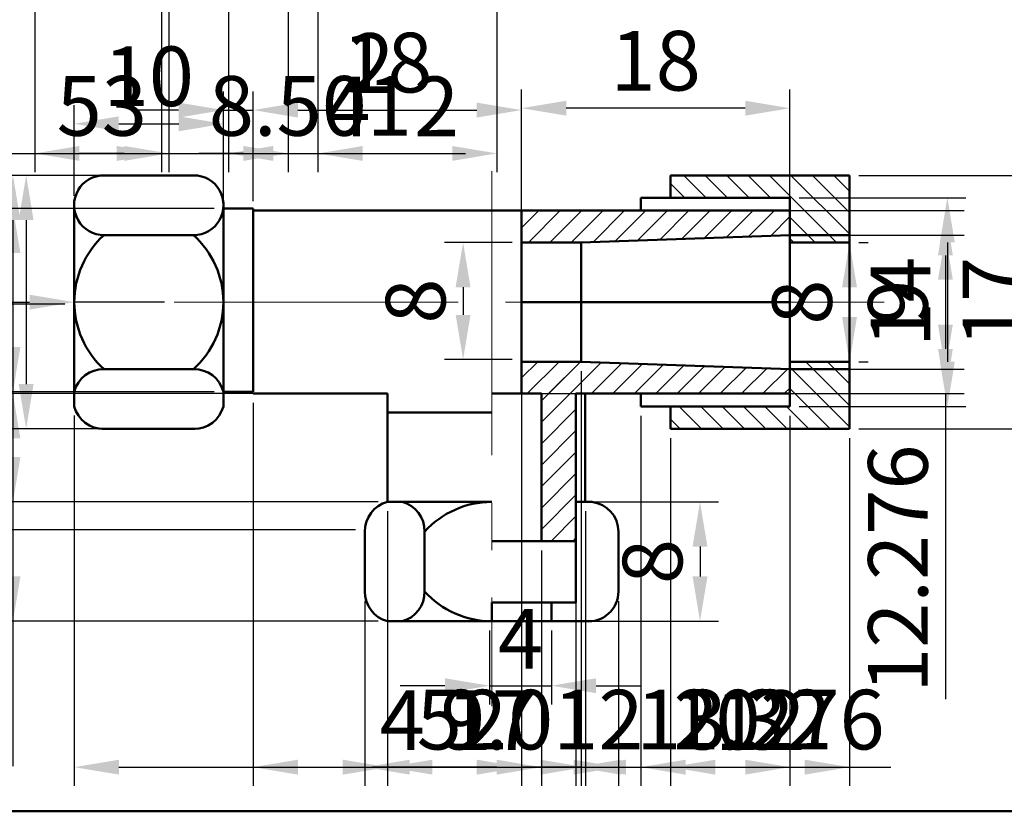
# Model space of a CAD drawing. Units: millimetres. Extents: x 139 to 291, y 28 to 164.
# Tile 2 of 5: x 174 to 240, y 28 to 81. Entities that reach past the tile are written whole.
import ezdxf

# ---------------------------------------------------------------- set-up
doc = ezdxf.new("R2010")
doc.units = ezdxf.units.MM
doc.linetypes.add('CENTER2', pattern=[28.575, 19.05, -3.175, 3.175, -3.175])
for name, color, linetype, lineweight in [('M-CNTR', 1, 'CENTER2', 18), ('M-DIMS', 2, 'Continuous', 25), ('M-HATC', 8, 'Continuous', 18), ('M-OUTL', 7, 'Continuous', 50)]:
    doc.layers.add(name, color=color, linetype=linetype, lineweight=lineweight)
doc.styles.get("Standard").update_dxf_attribs({"font": 'arial.ttf'})
doc.dimstyles.new('ISO-25', dxfattribs={"dimtxt": 4, "dimasz": 3, "dimexe": 1.25, "dimexo": 0.625, "dimtad": 1, "dimdec": 0, "dimtxsty": 'Standard', "dimcen": 2.5, "dimadec": 0, "dimazin": 0, "dimtfac": 1, "dimtdec": 0, "dimtmove": 0, "dimatfit": 3, "dimfxl": 1, "dimarcsym": 0})
pattern_1 = [(45, (183.714, -20.9195), (-0.71842, 0.71842), [])]

# ---------------------------------------------------------------- blocks, each defined once
blk = doc.blocks.new('*D26')
at = {"layer": 'Defpoints', "color": 0, "transparency": 16777216}
for p in [(187.298, 74.293), (177.276, 68.836), (187.298, 68.836)]:
    blk.add_point(p, dxfattribs=at)
at = {"layer": 'M-DIMS', "color": 0, "lineweight": -2, "transparency": 16777216}
for p, q in [((177.276, 69.461), (177.276, 75.543)), ((187.298, 69.461), (187.298, 75.543)), ((180.276, 74.293), (184.298, 74.293))]:
    blk.add_line(p, q, dxfattribs=at)
at = {"layer": 'M-DIMS', "color": 0, "transparency": 16777216}
for points in [[(180.276, 74.793), (180.276, 73.793), (177.276, 74.293)], [(184.298, 74.793), (184.298, 73.793), (187.298, 74.293)]]:
    blk.add_solid(points, dxfattribs=at)
at = {"layer": 'M-DIMS', "color": 0, "transparency": 16777216, "insert": (182.287, 76.96), "char_height": 4, "attachment_point": 5}
blk.add_mtext('10', dxfattribs=at)
blk = doc.blocks.new('*D27')
at = {"layer": 'Defpoints', "color": 0, "transparency": 16777216}
for p in [(180.776, 70.836), (174.061, 53.836), (180.776, 53.836)]:
    blk.add_point(p, dxfattribs=at)
at = {"layer": 'M-DIMS', "color": 0, "lineweight": -2, "transparency": 16777216}
for p, q in [((180.151, 70.836), (172.811, 70.836)), ((174.061, 67.836), (174.061, 56.836)), ((180.151, 53.836), (172.811, 53.836))]:
    blk.add_line(p, q, dxfattribs=at)
at = {"layer": 'M-DIMS', "color": 0, "transparency": 16777216}
for points in [[(173.561, 67.836), (174.561, 67.836), (174.061, 70.836)], [(173.561, 56.836), (174.561, 56.836), (174.061, 53.836)]]:
    blk.add_solid(points, dxfattribs=at)
at = {"layer": 'M-DIMS', "color": 0, "transparency": 16777216, "insert": (171.428, 62.336), "char_height": 4, "attachment_point": 5, "rotation": 90}
blk.add_mtext('17', dxfattribs=at)
blk = doc.blocks.new('*D28')
at = {"layer": 'Defpoints', "color": 0, "transparency": 16777216}
for p in [(177.287, 62.199), (167.49, 47.061), (196.787, 47.061)]:
    blk.add_point(p, dxfattribs=at)
at = {"layer": 'M-DIMS', "color": 0, "lineweight": -2, "transparency": 16777216}
for p, q in [((176.662, 62.199), (166.24, 62.199)), ((167.49, 59.199), (167.49, 50.061)), ((196.162, 47.061), (166.24, 47.061))]:
    blk.add_line(p, q, dxfattribs=at)
at = {"layer": 'M-DIMS', "color": 0, "transparency": 16777216}
for points in [[(166.99, 59.199), (167.99, 59.199), (167.49, 62.199)], [(166.99, 50.061), (167.99, 50.061), (167.49, 47.061)]]:
    blk.add_solid(points, dxfattribs=at)
at = {"layer": 'M-DIMS', "color": 0, "transparency": 16777216, "insert": (164.822, 54.63), "char_height": 4, "attachment_point": 5, "rotation": 90}
blk.add_mtext('15', dxfattribs=at)
blk = doc.blocks.new('*D29')
at = {"layer": 'Defpoints', "color": 0, "transparency": 16777216}
for p in [(211.561, 48.942), (211.469, 40.942), (219.258, 40.942)]:
    blk.add_point(p, dxfattribs=at)
at = {"layer": 'M-DIMS', "color": 0, "lineweight": -2, "transparency": 16777216}
for p, q in [((212.186, 48.942), (220.508, 48.942)), ((219.258, 45.942), (219.258, 43.942)), ((212.094, 40.942), (220.508, 40.942))]:
    blk.add_line(p, q, dxfattribs=at)
at = {"layer": 'M-DIMS', "color": 0, "transparency": 16777216}
for points in [[(218.758, 45.942), (219.758, 45.942), (219.258, 48.942)], [(218.758, 43.942), (219.758, 43.942), (219.258, 40.942)]]:
    blk.add_solid(points, dxfattribs=at)
at = {"layer": 'M-DIMS', "color": 0, "transparency": 16777216, "insert": (216.591, 44.942), "char_height": 4, "attachment_point": 5, "rotation": 90}
blk.add_mtext('8', dxfattribs=at)
blk = doc.blocks.new('*D30')
at = {"layer": 'Defpoints', "color": 0, "transparency": 16777216}
for p in [(205.149, 40.942), (209.287, 40.942), (209.287, 36.614)]:
    blk.add_point(p, dxfattribs=at)
at = {"layer": 'M-DIMS', "color": 0, "lineweight": -2, "transparency": 16777216}
for p, q in [((205.149, 40.317), (205.149, 35.364)), ((209.287, 40.317), (209.287, 35.364)), ((202.149, 36.614), (199.149, 36.614)), ((205.149, 36.614), (209.287, 36.614)), ((212.287, 36.614), (215.287, 36.614))]:
    blk.add_line(p, q, dxfattribs=at)
at = {"layer": 'M-DIMS', "color": 0, "transparency": 16777216}
for points in [[(202.149, 37.114), (202.149, 36.114), (205.149, 36.614)], [(212.287, 37.114), (212.287, 36.114), (209.287, 36.614)]]:
    blk.add_solid(points, dxfattribs=at)
at = {"layer": 'M-DIMS', "color": 0, "transparency": 16777216, "insert": (207.218, 39.239), "char_height": 4, "attachment_point": 5}
blk.add_mtext('4', dxfattribs=at)
blk = doc.blocks.new('*D31')
at = {"layer": 'Defpoints', "color": 0, "transparency": 16777216}
for p in [(229.287, 70.836), (229.287, 53.836), (242.032, 53.836)]:
    blk.add_point(p, dxfattribs=at)
at = {"layer": 'M-DIMS', "color": 0, "lineweight": -2, "transparency": 16777216}
for p, q in [((229.912, 70.836), (243.282, 70.836)), ((242.032, 67.836), (242.032, 56.836)), ((229.912, 53.836), (243.282, 53.836))]:
    blk.add_line(p, q, dxfattribs=at)
at = {"layer": 'M-DIMS', "color": 0, "transparency": 16777216}
for points in [[(241.532, 67.836), (242.532, 67.836), (242.032, 70.836)], [(241.532, 56.836), (242.532, 56.836), (242.032, 53.836)]]:
    blk.add_solid(points, dxfattribs=at)
at = {"layer": 'M-DIMS', "color": 0, "transparency": 16777216, "insert": (239.399, 62.336), "char_height": 4, "attachment_point": 5, "rotation": 90}
blk.add_mtext('17', dxfattribs=at)
blk = doc.blocks.new('*D32')
at = {"layer": 'Defpoints', "color": 0, "transparency": 16777216}
for p in [(225.287, 69.336), (225.287, 55.336), (235.847, 55.336)]:
    blk.add_point(p, dxfattribs=at)
at = {"layer": 'M-DIMS', "color": 0, "lineweight": -2, "transparency": 16777216}
for p, q in [((225.912, 69.336), (237.097, 69.336)), ((235.847, 66.336), (235.847, 58.336)), ((225.912, 55.336), (237.097, 55.336))]:
    blk.add_line(p, q, dxfattribs=at)
at = {"layer": 'M-DIMS', "color": 0, "transparency": 16777216}
for points in [[(235.347, 66.336), (236.347, 66.336), (235.847, 69.336)], [(235.347, 58.336), (236.347, 58.336), (235.847, 55.336)]]:
    blk.add_solid(points, dxfattribs=at)
at = {"layer": 'M-DIMS', "color": 0, "transparency": 16777216, "insert": (233.214, 62.336), "char_height": 4, "attachment_point": 5, "rotation": 90}
blk.add_mtext('14', dxfattribs=at)
blk = doc.blocks.new('*D33')
at = {"layer": 'Defpoints', "color": 0, "transparency": 16777216}
for p in [(229.287, 66.336), (229.287, 58.336), (229.287, 58.336)]:
    blk.add_point(p, dxfattribs=at)
at = {"layer": 'M-DIMS', "color": 0, "lineweight": -2, "transparency": 16777216}
for p, q in [((229.912, 66.336), (230.537, 66.336)), ((229.287, 63.336), (229.287, 61.336)), ((229.912, 58.336), (230.537, 58.336))]:
    blk.add_line(p, q, dxfattribs=at)
at = {"layer": 'M-DIMS', "color": 0, "transparency": 16777216}
for points in [[(228.787, 63.336), (229.787, 63.336), (229.287, 66.336)], [(228.787, 61.336), (229.787, 61.336), (229.287, 58.336)]]:
    blk.add_solid(points, dxfattribs=at)
at = {"layer": 'M-DIMS', "color": 0, "transparency": 16777216, "insert": (226.62, 62.336), "char_height": 4, "attachment_point": 5, "rotation": 90}
blk.add_mtext('8', dxfattribs=at)
blk = doc.blocks.new('*D34')
at = {"layer": 'Defpoints', "color": 0, "transparency": 16777216}
for p in [(207.287, 66.336), (203.367, 58.479), (207.287, 58.479)]:
    blk.add_point(p, dxfattribs=at)
at = {"layer": 'M-DIMS', "color": 0, "lineweight": -2, "transparency": 16777216}
for p, q in [((206.662, 66.336), (202.117, 66.336)), ((203.367, 63.336), (203.367, 61.479)), ((206.662, 58.479), (202.117, 58.479))]:
    blk.add_line(p, q, dxfattribs=at)
at = {"layer": 'M-DIMS', "color": 0, "transparency": 16777216}
for points in [[(202.867, 63.336), (203.867, 63.336), (203.367, 66.336)], [(202.867, 61.479), (203.867, 61.479), (203.367, 58.479)]]:
    blk.add_solid(points, dxfattribs=at)
at = {"layer": 'M-DIMS', "color": 0, "transparency": 16777216, "insert": (200.7, 62.408), "char_height": 4, "attachment_point": 5, "rotation": 90}
blk.add_mtext('8', dxfattribs=at)
blk = doc.blocks.new('*D35')
at = {"layer": 'Defpoints', "color": 0, "transparency": 16777216}
for p in [(207.287, 75.339), (207.287, 62.336), (225.287, 62.336)]:
    blk.add_point(p, dxfattribs=at)
at = {"layer": 'M-DIMS', "color": 0, "lineweight": -2, "transparency": 16777216}
for p, q in [((207.287, 62.961), (207.287, 76.589)), ((225.287, 62.961), (225.287, 76.589)), ((222.287, 75.339), (210.287, 75.339))]:
    blk.add_line(p, q, dxfattribs=at)
at = {"layer": 'M-DIMS', "color": 0, "transparency": 16777216}
for points in [[(210.287, 75.839), (210.287, 74.839), (207.287, 75.339)], [(222.287, 75.839), (222.287, 74.839), (225.287, 75.339)]]:
    blk.add_solid(points, dxfattribs=at)
at = {"layer": 'M-DIMS', "color": 0, "transparency": 16777216, "insert": (216.287, 78.006), "char_height": 4, "attachment_point": 5}
blk.add_mtext('18', dxfattribs=at)
blk = doc.blocks.new('*D36')
at = {"layer": 'Defpoints', "color": 0, "transparency": 16777216}
for p in [(152.636, 94.663), (205.636, 89.163), (205.636, 72.308)]:
    blk.add_point(p, dxfattribs=at)
at = {"layer": 'M-DIMS', "color": 0, "lineweight": -2, "transparency": 16777216}
for p, q in [((152.636, 94.038), (152.636, 71.058)), ((205.636, 88.538), (205.636, 71.058)), ((155.636, 72.308), (202.636, 72.308))]:
    blk.add_line(p, q, dxfattribs=at)
at = {"layer": 'M-DIMS', "color": 0, "transparency": 16777216}
for points in [[(155.636, 72.808), (155.636, 71.808), (152.636, 72.308)], [(202.636, 72.808), (202.636, 71.808), (205.636, 72.308)]]:
    blk.add_solid(points, dxfattribs=at)
at = {"layer": 'M-DIMS', "color": 0, "transparency": 16777216, "insert": (179.136, 74.977), "char_height": 4, "attachment_point": 5}
blk.add_mtext('53', dxfattribs=at)
blk = doc.blocks.new('*D37')
at = {"layer": 'Defpoints', "color": 0, "transparency": 16777216}
for p in [(174.636, 99.163), (183.137, 99.163), (183.137, 72.308)]:
    blk.add_point(p, dxfattribs=at)
at = {"layer": 'M-DIMS', "color": 0, "lineweight": -2, "transparency": 16777216}
for p, q in [((174.636, 98.538), (174.636, 71.058)), ((183.137, 98.538), (183.137, 71.058)), ((177.636, 72.308), (180.137, 72.308)), ((183.137, 72.308), (200.118, 72.308))]:
    blk.add_line(p, q, dxfattribs=at)
at = {"layer": 'M-DIMS', "color": 0, "transparency": 16777216}
for points in [[(177.636, 72.808), (177.636, 71.808), (174.636, 72.308)], [(180.137, 72.808), (180.137, 71.808), (183.137, 72.308)]]:
    blk.add_solid(points, dxfattribs=at)
at = {"layer": 'M-DIMS', "color": 0, "transparency": 16777216, "insert": (193.128, 74.976), "char_height": 4, "attachment_point": 5}
blk.add_mtext('8.501', dxfattribs=at)
blk = doc.blocks.new('*D38')
at = {"layer": 'Defpoints', "color": 0, "transparency": 16777216}
for p in [(187.636, 101.663), (183.636, 97.663), (187.636, 72.308)]:
    blk.add_point(p, dxfattribs=at)
at = {"layer": 'M-DIMS', "color": 0, "lineweight": -2, "transparency": 16777216}
for p, q in [((187.636, 101.038), (187.636, 71.058)), ((183.636, 97.038), (183.636, 71.058)), ((180.636, 72.308), (177.636, 72.308)), ((183.636, 72.308), (187.636, 72.308)), ((190.636, 72.308), (197.653, 72.308))]:
    blk.add_line(p, q, dxfattribs=at)
at = {"layer": 'M-DIMS', "color": 0, "transparency": 16777216}
for points in [[(180.636, 72.808), (180.636, 71.808), (183.636, 72.308)], [(190.636, 72.808), (190.636, 71.808), (187.636, 72.308)]]:
    blk.add_solid(points, dxfattribs=at)
at = {"layer": 'M-DIMS', "color": 0, "transparency": 16777216, "insert": (195.644, 74.933), "char_height": 4, "attachment_point": 5}
blk.add_mtext('4', dxfattribs=at)
blk = doc.blocks.new('*D41')
at = {"layer": 'Defpoints', "color": 0, "transparency": 16777216}
for p in [(191.636, 104.663), (193.636, 104.663), (193.636, 72.308)]:
    blk.add_point(p, dxfattribs=at)
at = {"layer": 'M-DIMS', "color": 0, "lineweight": -2, "transparency": 16777216}
for p, q in [((191.636, 104.038), (191.636, 71.058)), ((193.636, 104.038), (193.636, 71.058)), ((188.636, 72.308), (185.636, 72.308)), ((191.636, 72.308), (193.636, 72.308)), ((196.636, 72.308), (203.535, 72.308))]:
    blk.add_line(p, q, dxfattribs=at)
at = {"layer": 'M-DIMS', "color": 0, "transparency": 16777216}
for points in [[(188.636, 72.808), (188.636, 71.808), (191.636, 72.308)], [(196.636, 72.808), (196.636, 71.808), (193.636, 72.308)]]:
    blk.add_solid(points, dxfattribs=at)
at = {"layer": 'M-DIMS', "color": 0, "transparency": 16777216, "insert": (201.586, 74.942), "char_height": 4, "attachment_point": 5}
blk.add_mtext('2', dxfattribs=at)
blk = doc.blocks.new('*D42')
at = {"layer": 'Defpoints', "color": 0, "transparency": 16777216}
for p in [(177.287, 55.349), (229.287, 53.836), (229.287, 31.154)]:
    blk.add_point(p, dxfattribs=at)
at = {"layer": 'M-DIMS', "color": 0, "lineweight": -2, "transparency": 16777216}
for p, q in [((177.287, 54.724), (177.287, 29.904)), ((229.287, 53.211), (229.287, 29.904)), ((180.287, 31.154), (226.287, 31.154))]:
    blk.add_line(p, q, dxfattribs=at)
at = {"layer": 'M-DIMS', "color": 0, "transparency": 16777216}
for points in [[(180.287, 31.654), (180.287, 30.654), (177.287, 31.154)], [(226.287, 31.654), (226.287, 30.654), (229.287, 31.154)]]:
    blk.add_solid(points, dxfattribs=at)
at = {"layer": 'M-DIMS', "color": 0, "transparency": 16777216, "insert": (203.287, 33.822), "char_height": 4, "attachment_point": 5}
blk.add_mtext('52', dxfattribs=at)
blk = doc.blocks.new('*D43')
at = {"layer": 'Defpoints', "color": 0, "transparency": 16777216}
for p in [(179.287, 70.836), (173.176, 40.942), (198.299, 40.942)]:
    blk.add_point(p, dxfattribs=at)
at = {"layer": 'M-DIMS', "color": 0, "lineweight": -2, "transparency": 16777216}
for p, q in [((178.662, 70.836), (171.926, 70.836)), ((173.176, 67.836), (173.176, 43.942)), ((197.674, 40.942), (171.926, 40.942))]:
    blk.add_line(p, q, dxfattribs=at)
at = {"layer": 'M-DIMS', "color": 0, "transparency": 16777216}
for points in [[(172.676, 67.836), (173.676, 67.836), (173.176, 70.836)], [(172.676, 43.942), (173.676, 43.942), (173.176, 40.942)]]:
    blk.add_solid(points, dxfattribs=at)
at = {"layer": 'M-DIMS', "color": 0, "transparency": 16777216, "insert": (170.509, 55.889), "char_height": 4, "attachment_point": 5, "rotation": 90}
blk.add_mtext('29.895', dxfattribs=at)
blk = doc.blocks.new('*D44')
at = {"layer": 'Defpoints', "color": 0, "transparency": 16777216}
for p in [(207.287, 68.474), (207.287, 56.199), (235.718, 56.199)]:
    blk.add_point(p, dxfattribs=at)
at = {"layer": 'M-DIMS', "color": 0, "lineweight": -2, "transparency": 16777216}
for p, q in [((207.912, 68.474), (236.968, 68.474)), ((235.718, 65.474), (235.718, 59.199)), ((207.912, 56.199), (236.968, 56.199)), ((235.718, 56.199), (235.718, 35.722))]:
    blk.add_line(p, q, dxfattribs=at)
at = {"layer": 'M-DIMS', "color": 0, "transparency": 16777216}
for points in [[(235.218, 65.474), (236.218, 65.474), (235.718, 68.474)], [(235.218, 59.199), (236.218, 59.199), (235.718, 56.199)]]:
    blk.add_solid(points, dxfattribs=at)
at = {"layer": 'M-DIMS', "color": 0, "transparency": 16777216, "insert": (233.051, 44.46), "char_height": 4, "attachment_point": 5, "rotation": 90}
blk.add_mtext('12.276', dxfattribs=at)
blk = doc.blocks.new('*D45')
at = {"layer": 'Defpoints', "color": 0, "transparency": 16777216}
for p in [(189.287, 75.214), (187.287, 68.624), (189.287, 68.624)]:
    blk.add_point(p, dxfattribs=at)
at = {"layer": 'M-DIMS', "color": 0, "lineweight": -2, "transparency": 16777216}
for p, q in [((187.287, 69.249), (187.287, 76.464)), ((189.287, 69.249), (189.287, 76.464)), ((184.287, 75.214), (181.287, 75.214)), ((187.287, 75.214), (189.287, 75.214)), ((192.287, 75.214), (199.187, 75.214))]:
    blk.add_line(p, q, dxfattribs=at)
at = {"layer": 'M-DIMS', "color": 0, "transparency": 16777216}
for points in [[(184.287, 75.714), (184.287, 74.714), (187.287, 75.214)], [(192.287, 75.714), (192.287, 74.714), (189.287, 75.214)]]:
    blk.add_solid(points, dxfattribs=at)
at = {"layer": 'M-DIMS', "color": 0, "transparency": 16777216, "insert": (197.237, 77.847), "char_height": 4, "attachment_point": 5}
blk.add_mtext('2', dxfattribs=at)
blk = doc.blocks.new('*D46')
at = {"layer": 'Defpoints', "color": 0, "transparency": 16777216}
for p in [(187.287, 68.624), (173.176, 56.324), (187.287, 56.324)]:
    blk.add_point(p, dxfattribs=at)
at = {"layer": 'M-DIMS', "color": 0, "lineweight": -2, "transparency": 16777216}
for p, q in [((186.662, 68.624), (171.926, 68.624)), ((173.176, 65.624), (173.176, 59.324)), ((186.662, 56.324), (171.926, 56.324))]:
    blk.add_line(p, q, dxfattribs=at)
at = {"layer": 'M-DIMS', "color": 0, "transparency": 16777216}
for points in [[(172.676, 65.624), (173.676, 65.624), (173.176, 68.624)], [(172.676, 59.324), (173.676, 59.324), (173.176, 56.324)]]:
    blk.add_solid(points, dxfattribs=at)
at = {"layer": 'M-DIMS', "color": 0, "transparency": 16777216, "insert": (170.507, 62.474), "char_height": 4, "attachment_point": 5, "rotation": 90}
blk.add_mtext('12.3', dxfattribs=at)
blk = doc.blocks.new('*D47')
at = {"layer": 'Defpoints', "color": 0, "transparency": 16777216}
for p in [(207.287, 75.214), (189.287, 68.474), (207.287, 68.474)]:
    blk.add_point(p, dxfattribs=at)
at = {"layer": 'M-DIMS', "color": 0, "lineweight": -2, "transparency": 16777216}
for p, q in [((189.287, 69.099), (189.287, 76.464)), ((207.287, 69.099), (207.287, 76.464)), ((192.287, 75.214), (204.287, 75.214))]:
    blk.add_line(p, q, dxfattribs=at)
at = {"layer": 'M-DIMS', "color": 0, "transparency": 16777216}
for points in [[(192.287, 75.714), (192.287, 74.714), (189.287, 75.214)], [(204.287, 75.714), (204.287, 74.714), (207.287, 75.214)]]:
    blk.add_solid(points, dxfattribs=at)
at = {"layer": 'M-DIMS', "color": 0, "transparency": 16777216, "insert": (198.287, 77.881), "char_height": 4, "attachment_point": 5}
blk.add_mtext('18', dxfattribs=at)
blk = doc.blocks.new('*D48')
at = {"layer": 'Defpoints', "color": 0, "transparency": 16777216}
for p in [(189.287, 56.199), (198.299, 48.942), (198.299, 31.154)]:
    blk.add_point(p, dxfattribs=at)
at = {"layer": 'M-DIMS', "color": 0, "lineweight": -2, "transparency": 16777216}
for p, q in [((189.287, 55.574), (189.287, 29.904)), ((198.299, 48.317), (198.299, 29.904)), ((192.287, 31.154), (195.299, 31.154)), ((198.299, 31.154), (216.006, 31.154))]:
    blk.add_line(p, q, dxfattribs=at)
at = {"layer": 'M-DIMS', "color": 0, "transparency": 16777216}
for points in [[(192.287, 31.654), (192.287, 30.654), (189.287, 31.154)], [(195.299, 31.654), (195.299, 30.654), (198.299, 31.154)]]:
    blk.add_solid(points, dxfattribs=at)
at = {"layer": 'M-DIMS', "color": 0, "transparency": 16777216, "insert": (208.653, 33.822), "char_height": 4, "attachment_point": 5}
blk.add_mtext('9.012', dxfattribs=at)
blk = doc.blocks.new('*D49')
at = {"layer": 'Defpoints', "color": 0, "transparency": 16777216}
for p in [(198.299, 48.942), (211.575, 48.942), (211.575, 31.154)]:
    blk.add_point(p, dxfattribs=at)
at = {"layer": 'M-DIMS', "color": 0, "lineweight": -2, "transparency": 16777216}
for p, q in [((198.299, 48.317), (198.299, 29.904)), ((211.575, 48.317), (211.575, 29.904)), ((201.299, 31.154), (208.575, 31.154)), ((211.575, 31.154), (232.051, 31.154))]:
    blk.add_line(p, q, dxfattribs=at)
at = {"layer": 'M-DIMS', "color": 0, "transparency": 16777216}
for points in [[(201.299, 31.654), (201.299, 30.654), (198.299, 31.154)], [(208.575, 31.654), (208.575, 30.654), (211.575, 31.154)]]:
    blk.add_solid(points, dxfattribs=at)
at = {"layer": 'M-DIMS', "color": 0, "transparency": 16777216, "insert": (223.313, 33.823), "char_height": 4, "attachment_point": 5}
blk.add_mtext('13.276', dxfattribs=at)
blk = doc.blocks.new('*D50')
at = {"layer": 'Defpoints', "color": 0, "transparency": 16777216}
for p in [(198.299, 56.199), (173.176, 48.942), (198.299, 48.942)]:
    blk.add_point(p, dxfattribs=at)
at = {"layer": 'M-DIMS', "color": 0, "lineweight": -2, "transparency": 16777216}
for p, q in [((197.674, 56.199), (171.926, 56.199)), ((173.176, 53.199), (173.176, 51.942)), ((197.674, 48.942), (171.926, 48.942)), ((173.176, 48.942), (173.176, 31.227))]:
    blk.add_line(p, q, dxfattribs=at)
at = {"layer": 'M-DIMS', "color": 0, "transparency": 16777216}
for points in [[(172.676, 53.199), (173.676, 53.199), (173.176, 56.199)], [(172.676, 51.942), (173.676, 51.942), (173.176, 48.942)]]:
    blk.add_solid(points, dxfattribs=at)
at = {"layer": 'M-DIMS', "color": 0, "transparency": 16777216, "insert": (170.509, 38.584), "char_height": 4, "attachment_point": 5, "rotation": 90}
blk.add_mtext('7.257', dxfattribs=at)
blk = doc.blocks.new('*D51')
at = {"layer": 'Defpoints', "color": 0, "transparency": 16777216}
for p in [(196.787, 42.942), (213.787, 42.919), (213.787, 31.154)]:
    blk.add_point(p, dxfattribs=at)
at = {"layer": 'M-DIMS', "color": 0, "lineweight": -2, "transparency": 16777216}
for p, q in [((196.787, 42.317), (196.787, 29.904)), ((213.787, 42.294), (213.787, 29.904)), ((199.787, 31.154), (210.787, 31.154))]:
    blk.add_line(p, q, dxfattribs=at)
at = {"layer": 'M-DIMS', "color": 0, "transparency": 16777216}
for points in [[(199.787, 31.654), (199.787, 30.654), (196.787, 31.154)], [(210.787, 31.654), (210.787, 30.654), (213.787, 31.154)]]:
    blk.add_solid(points, dxfattribs=at)
at = {"layer": 'M-DIMS', "color": 0, "transparency": 16777216, "insert": (205.287, 33.788), "char_height": 4, "attachment_point": 5}
blk.add_mtext('17', dxfattribs=at)
blk = doc.blocks.new('*D52')
at = {"layer": 'Defpoints', "color": 0, "transparency": 16777216}
for p in [(208.623, 46.316), (210.938, 46.316), (210.938, 31.154)]:
    blk.add_point(p, dxfattribs=at)
at = {"layer": 'M-DIMS', "color": 0, "lineweight": -2, "transparency": 16777216}
for p, q in [((208.623, 45.691), (208.623, 29.904)), ((210.938, 45.691), (210.938, 29.904)), ((205.623, 31.154), (202.623, 31.154)), ((208.623, 31.154), (210.938, 31.154)), ((213.938, 31.154), (228.606, 31.154))]:
    blk.add_line(p, q, dxfattribs=at)
at = {"layer": 'M-DIMS', "color": 0, "transparency": 16777216}
for points in [[(205.623, 31.654), (205.623, 30.654), (208.623, 31.154)], [(213.938, 31.654), (213.938, 30.654), (210.938, 31.154)]]:
    blk.add_solid(points, dxfattribs=at)
at = {"layer": 'M-DIMS', "color": 0, "transparency": 16777216, "insert": (222.772, 33.823), "char_height": 4, "attachment_point": 5}
blk.add_mtext('2.32', dxfattribs=at)
blk = doc.blocks.new('*D53')
at = {"layer": 'Defpoints', "color": 0, "transparency": 16777216}
for p in [(215.287, 55.336), (225.287, 55.336), (225.287, 31.154)]:
    blk.add_point(p, dxfattribs=at)
at = {"layer": 'M-DIMS', "color": 0, "lineweight": -2, "transparency": 16777216}
for p, q in [((215.287, 54.711), (215.287, 29.904)), ((225.287, 54.711), (225.287, 29.904)), ((218.287, 31.154), (222.287, 31.154))]:
    blk.add_line(p, q, dxfattribs=at)
at = {"layer": 'M-DIMS', "color": 0, "transparency": 16777216}
for points in [[(218.287, 31.654), (218.287, 30.654), (215.287, 31.154)], [(222.287, 31.654), (222.287, 30.654), (225.287, 31.154)]]:
    blk.add_solid(points, dxfattribs=at)
at = {"layer": 'M-DIMS', "color": 0, "transparency": 16777216, "insert": (220.287, 33.822), "char_height": 4, "attachment_point": 5}
blk.add_mtext('10', dxfattribs=at)
blk = doc.blocks.new('*D54')
at = {"layer": 'Defpoints', "color": 0, "transparency": 16777216}
for p in [(217.287, 53.836), (229.287, 53.836), (229.287, 31.154)]:
    blk.add_point(p, dxfattribs=at)
at = {"layer": 'M-DIMS', "color": 0, "lineweight": -2, "transparency": 16777216}
for p, q in [((217.287, 53.211), (217.287, 29.904)), ((229.287, 53.211), (229.287, 29.904)), ((220.287, 31.154), (226.287, 31.154))]:
    blk.add_line(p, q, dxfattribs=at)
at = {"layer": 'M-DIMS', "color": 0, "transparency": 16777216}
for points in [[(220.287, 31.654), (220.287, 30.654), (217.287, 31.154)], [(226.287, 31.654), (226.287, 30.654), (229.287, 31.154)]]:
    blk.add_solid(points, dxfattribs=at)
at = {"layer": 'M-DIMS', "color": 0, "transparency": 16777216, "insert": (223.287, 33.788), "char_height": 4, "attachment_point": 5}
blk.add_mtext('12', dxfattribs=at)
blk = doc.blocks.new('*D55')
at = {"layer": 'Defpoints', "color": 0, "transparency": 16777216}
for p in [(207.287, 58.336), (211.287, 58.336), (207.287, 31.154)]:
    blk.add_point(p, dxfattribs=at)
at = {"layer": 'M-DIMS', "color": 0, "lineweight": -2, "transparency": 16777216}
for p, q in [((207.287, 57.711), (207.287, 29.904)), ((211.287, 57.711), (211.287, 29.904)), ((204.287, 31.154), (197.27, 31.154)), ((211.287, 31.154), (207.287, 31.154)), ((214.287, 31.154), (217.287, 31.154))]:
    blk.add_line(p, q, dxfattribs=at)
at = {"layer": 'M-DIMS', "color": 0, "transparency": 16777216}
for points in [[(204.287, 31.654), (204.287, 30.654), (207.287, 31.154)], [(214.287, 31.654), (214.287, 30.654), (211.287, 31.154)]]:
    blk.add_solid(points, dxfattribs=at)
at = {"layer": 'M-DIMS', "color": 0, "transparency": 16777216, "insert": (199.279, 33.779), "char_height": 4, "attachment_point": 5}
blk.add_mtext('4', dxfattribs=at)
blk = doc.blocks.new('*D56')
at = {"layer": 'Defpoints', "color": 0, "transparency": 16777216}
for p in [(225.287, 66.836), (225.287, 57.836), (235.718, 57.836)]:
    blk.add_point(p, dxfattribs=at)
at = {"layer": 'M-DIMS', "color": 0, "lineweight": -2, "transparency": 16777216}
for p, q in [((225.912, 66.836), (236.968, 66.836)), ((235.718, 63.836), (235.718, 60.836)), ((225.912, 57.836), (236.968, 57.836))]:
    blk.add_line(p, q, dxfattribs=at)
at = {"layer": 'M-DIMS', "color": 0, "transparency": 16777216}
for points in [[(235.218, 63.836), (236.218, 63.836), (235.718, 66.836)], [(235.218, 60.836), (236.218, 60.836), (235.718, 57.836)]]:
    blk.add_solid(points, dxfattribs=at)
at = {"layer": 'M-DIMS', "color": 0, "transparency": 16777216, "insert": (233.051, 62.336), "char_height": 4, "attachment_point": 5, "rotation": 90}
blk.add_mtext('9', dxfattribs=at)
blk = doc.blocks.new('*D60')
at = {"layer": 'Defpoints', "color": 0, "transparency": 16777216}
for p in [(177.287, 62.336), (183.35, 62.336)]:
    blk.add_point(p, dxfattribs=at)
at = {"layer": 'M-DIMS', "color": 0, "lineweight": -2, "transparency": 16777216}
for p, q in [((152.711, 62.334), (174.287, 62.336)), ((183.35, 62.336), (177.287, 62.336))]:
    blk.add_line(p, q, dxfattribs=at)
at = {"layer": 'M-DIMS', "color": 0, "transparency": 16777216}
blk.add_solid([(174.287, 62.836), (174.287, 61.836), (177.287, 62.336)], dxfattribs=at)
at = {"layer": 'M-DIMS', "color": 0, "transparency": 16777216, "insert": (161.999, 65.004), "char_height": 4, "attachment_point": 5, "rotation": 0.00419}
blk.add_mtext('R6.063', dxfattribs=at)

msp = doc.modelspace()

# ---------------------------------------------------------------- hatches: boundary and pattern name
at = {"layer": 'M-HATC'}
h = msp.add_hatch(dxfattribs=at)
h.set_pattern_fill('ANSI31', color=256, scale=0.32, angle=90)
h.set_pattern_definition([(135, (23.6513, -43.5646), (-0.7184205, -0.7184205), [])])
h.paths.add_polyline_path([(229.2871, 70.8364), (217.2871, 70.8364), (217.2871, 69.3364), (225.2871, 69.3364), (225.2871, 66.8364), (229.2871, 66.8364)])
h.paths.add_polyline_path([(229.2871, 66.8364), (225.2871, 66.8364), (225.2871, 66.3364), (229.2871, 66.3364)])
h.paths.add_polyline_path([(229.2871, 57.8364), (225.2871, 57.8364), (225.2871, 55.3364), (217.2871, 55.3364), (217.2871, 53.8364), (229.2871, 53.8364)])
h.paths.add_polyline_path([(229.2871, 58.3364), (225.2871, 58.3364), (225.2871, 57.8364), (229.2871, 57.8364)])
h = msp.add_hatch(dxfattribs=at)
h.set_pattern_fill('ANSI31', color=256, scale=0.32)
h.set_pattern_definition(pattern_1)
h.paths.add_polyline_path([(225.2871, 68.4743), (211.2871, 68.4743), (211.2871, 66.3364), (225.2871, 66.8364)])
h.paths.add_polyline_path([(211.2871, 68.4743), (207.2871, 68.4743), (207.2871, 66.3364), (211.2871, 66.3364)])
h.paths.add_polyline_path([(211.2871, 58.3364), (207.2871, 58.3364), (207.2871, 56.1986), (211.2871, 56.1986)])
h.paths.add_polyline_path([(225.2871, 57.8364), (211.2871, 58.3364), (211.2871, 56.1986), (225.2871, 56.1986)])
h = msp.add_hatch(dxfattribs=at)
h.set_pattern_fill('ANSI31', color=256, scale=0.32)
h.set_pattern_definition(pattern_1)
h.paths.add_polyline_path([(210.9384, 56.1986), (225.2871, 56.1986), (225.2871, 57.8364), (211.2871, 58.3364), (207.2871, 58.3364), (207.2871, 56.1986), (208.6231, 56.1986), (208.6231, 46.3157), (210.9384, 46.3157)])

# ---------------------------------------------------------------- linework, layer by layer
at = {"layer": 'M-CNTR'}
for p, q in [((205.2871, 71.1136), (205.2871, 35.2545)), ((231.6179, 62.3364), (177.2871, 62.3364))]:
    msp.add_line(p, q, dxfattribs=at)
at = {"layer": 'M-OUTL'}
for p, q in [((182.2871, 70.8364), (179.2646, 70.8364)), ((185.3097, 70.8364), (182.2871, 70.8364)), ((217.2871, 69.3364), (217.2871, 70.8364)), ((217.2871, 70.8364), (229.2871, 70.8364)), ((229.2871, 62.3364), (229.2871, 70.8364)), ((177.2871, 69.0487), (177.2871, 55.3485)), ((187.2871, 55.3485), (187.2871, 69.0487)), ((225.2871, 69.3364), (215.2871, 69.3364)), ((215.2871, 69.3364), (215.2871, 68.4743)), ((225.2871, 66.8364), (225.2871, 69.3364)), ((177.2871, 68.1986), (177.3803, 68.1986)), ((187.2871, 68.6242), (189.2871, 68.6242)), ((189.2871, 68.6242), (189.2871, 56.3244)), ((189.2871, 62.4743), (189.2871, 68.4743)), ((189.2871, 68.4743), (225.2871, 68.4743)), ((207.2871, 56.1986), (207.2871, 68.4743)), ((182.2871, 66.8364), (179.2646, 66.8364)), ((185.3097, 66.8364), (182.2871, 66.8364)), ((211.2871, 66.3364), (225.2871, 66.8364)), ((225.2871, 66.8364), (229.2871, 66.8364)), ((225.2871, 66.3364), (225.2871, 66.8364)), ((211.2871, 66.3364), (207.2871, 66.3364)), ((207.2871, 66.3364), (207.2871, 58.4793)), ((211.2871, 62.3364), (211.2871, 66.3364)), ((225.2871, 66.3364), (229.2871, 66.3364)), ((225.2871, 66.3364), (225.2871, 58.3364)), ((225.2871, 62.3364), (207.2871, 62.3364)), ((211.2871, 62.3364), (211.2871, 58.3364)), ((229.2871, 62.3364), (229.2871, 53.8364)), ((211.2871, 58.3364), (207.2871, 58.3364)), ((211.2871, 58.3364), (225.2871, 57.8364)), ((225.2871, 58.3364), (229.2871, 58.3364)), ((225.2871, 57.8364), (225.2871, 58.3364)), ((182.2871, 57.8364), (179.1681, 57.8364)), ((185.4062, 57.8364), (182.2871, 57.8364)), ((225.2871, 57.8364), (229.2871, 57.8364)), ((225.2871, 57.8364), (225.2871, 55.3364)), ((189.2871, 56.3244), (187.2871, 56.3244)), ((189.2871, 56.1986), (198.2992, 56.1986)), ((198.2992, 48.9417), (198.2992, 56.1986)), ((205.2871, 56.1986), (208.6231, 56.1986)), ((208.6231, 56.1986), (208.6231, 46.3157)), ((210.9384, 46.3157), (210.9384, 56.1986)), ((210.9384, 56.1986), (225.2871, 56.1986)), ((211.5607, 48.9401), (211.5607, 56.1986)), ((215.2871, 55.8364), (215.2871, 56.1986)), ((215.2871, 55.3364), (215.2871, 55.8364)), ((198.2992, 54.9417), (205.2871, 54.9417)), ((225.2871, 55.3364), (215.2871, 55.3364)), ((217.2871, 53.8364), (217.2871, 55.3364)), ((179.1681, 53.8364), (182.2871, 53.8364)), ((182.2871, 53.8364), (185.4062, 53.8364)), ((229.2871, 53.8364), (217.2871, 53.8364)), ((205.2871, 48.9417), (198.2992, 48.9417)), ((211.9994, 48.9417), (210.9384, 48.9417)), ((196.7871, 47.0608), (196.7871, 44.9417)), ((200.7871, 44.9417), (200.7871, 47.0607)), ((213.7871, 44.9417), (213.7871, 46.9642)), ((205.2871, 46.3157), (210.9384, 46.3157)), ((210.9384, 46.3157), (210.9384, 42.1853)), ((196.7871, 44.9417), (196.7871, 42.8227)), ((200.7871, 42.8227), (200.7871, 44.9417)), ((213.7871, 42.9192), (213.7871, 44.9417)), ((210.9384, 42.1853), (205.2871, 42.1853)), ((205.2871, 42.1853), (205.2871, 40.9417)), ((209.2871, 42.1853), (209.2871, 40.9417)), ((198.2992, 40.9417), (211.9994, 40.9417)), ((207.2871, 40.9417), (207.2871, 40.9433))]:
    msp.add_line(p, q, dxfattribs=at)
msp.add_lwpolyline([(139.74, 164.2339), (291.244, 164.2339), (291.244, 28.1944), (139.74, 28.1944)], close=True, dxfattribs=at)
for centre, radius, start, end in [((179.2759, 68.8364), 2, 89.677332, 270.322668), ((185.2984, 68.8364), 2, 269.677332, 90.322668), ((183.3496, 62.3364), 6.0625, 132.075022, 227.924978), ((181.2246, 62.3364), 6.0625, 312.075022, 47.924978), ((179.2276, 55.8364), 2.0009, 88.295425, 165.885789), ((185.3467, 55.8364), 2.0009, 14.114211, 91.704575), ((179.2276, 55.8364), 2.0009, 194.114211, 271.70457), ((185.3467, 55.8364), 2.0009, 268.29543, 345.885789), ((198.7871, 47.0012), 2.0009, 104.114211, 181.70457), ((198.7871, 47.0012), 2.0009, 358.295425, 75.885789), ((205.2871, 42.8792), 6.0625, 90, 137.924978), ((211.7871, 46.953), 2, 96.092116, 96.50143), ((211.7871, 46.953), 2, 359.677332, 83.907884), ((198.7871, 42.8822), 2.0009, 178.29543, 255.885789), ((198.7871, 42.8822), 2.0009, 284.114211, 1.704575), ((205.2871, 47.0042), 6.0625, 222.075022, 270), ((211.7871, 42.9305), 2, 263.907884, 0.322668)]:
    msp.add_arc(centre, radius, start, end, dxfattribs=at)

# ---------------------------------------------------------------- dimensions: what is measured, and where the dimension line sits
at = {"layer": 'M-DIMS'}
for base, p1, p2, override, picture, middle in [((193.6359, 72.3085), (191.6359, 104.6632), (193.6359, 104.6632), {"dimdec": 0, "dimlfac": 1, "dimrnd": 0, "dimzin": 0, "dimdsep": 46, "dimlunit": 2}, '*D41', (201.5855, 74.9417)), ((187.6359, 72.3085), (183.6359, 97.6632), (187.6359, 101.6632), {"dimdec": 0, "dimlfac": 1, "dimrnd": 0, "dimzin": 0, "dimdsep": 46, "dimlunit": 2}, '*D38', (195.6442, 74.9335)), ((183.1373, 72.3085), (174.6359, 99.1632), (183.1373, 99.1632), {"dimdec": 3, "dimlfac": 1, "dimrnd": 0, "dimzin": 0, "dimdsep": 46, "dimlunit": 2}, '*D37', (193.1279, 74.9758)), ((205.6359, 72.3085), (152.6359, 94.6632), (205.6359, 89.1632), {"dimdec": 0, "dimlfac": 1, "dimrnd": 0, "dimzin": 0, "dimdsep": 46, "dimlunit": 2}, '*D36', (179.1359, 74.9771)), ((207.2871, 75.3385), (225.2871, 62.3364), (207.2871, 62.3364), {"dimclrd": 0, "dimclre": 0, "dimclrt": 0}, '*D35', (216.2871, 78.0058)), ((189.2871, 75.2136), (187.2871, 68.6242), (189.2871, 68.6242), {"dimdec": 0, "dimlfac": 1, "dimrnd": 0, "dimzin": 0, "dimdsep": 46, "dimlunit": 2}, '*D45', (197.2368, 77.8468)), ((207.2871, 75.2136), (189.2871, 68.4743), (207.2871, 68.4743), {"dimdec": 0, "dimlfac": 1, "dimrnd": 0, "dimzin": 0, "dimdsep": 46, "dimlunit": 2}, '*D47', (198.2871, 77.8809)), ((187.2984, 74.2927), (177.2758, 68.8364), (187.2984, 68.8364), {"dimclrd": 0, "dimclre": 0, "dimclrt": 0}, '*D26', (182.2871, 76.96)), ((207.2871, 31.1545), (211.2871, 58.3364), (207.2871, 58.3364), {"dimdec": 0, "dimlfac": 1, "dimrnd": 0, "dimzin": 0, "dimdsep": 46, "dimlunit": 2}, '*D55', (199.2788, 33.7795)), ((198.2992, 31.1545), (189.2871, 56.1986), (198.2992, 48.9417), {"dimdec": 3, "dimlfac": 1, "dimrnd": 0, "dimzin": 0, "dimdsep": 46, "dimlunit": 2}, '*D48', (208.6527, 33.8218)), ((229.2871, 31.1545), (177.2871, 55.3485), (229.2871, 53.8364), {"dimdec": 0, "dimlfac": 1, "dimrnd": 0, "dimzin": 0, "dimdsep": 46, "dimlunit": 2}, '*D42', (203.2871, 33.8218)), ((225.2871, 31.1545), (215.2871, 55.3364), (225.2871, 55.3364), {"dimdec": 0, "dimlfac": 1, "dimrnd": 0, "dimzin": 0, "dimdsep": 46, "dimlunit": 2}, '*D53', (220.2871, 33.8218)), ((229.2871, 31.1545), (217.2871, 53.8364), (229.2871, 53.8364), {"dimdec": 0, "dimlfac": 1, "dimrnd": 0, "dimzin": 0, "dimdsep": 46, "dimlunit": 2}, '*D54', (223.2871, 33.7877)), ((211.5749, 31.1545), (198.2992, 48.9417), (211.5749, 48.9417), {"dimdec": 3, "dimlfac": 1, "dimrnd": 0, "dimzin": 0, "dimdsep": 46, "dimlunit": 2}, '*D49', (223.3131, 33.8231)), ((210.9384, 31.1545), (208.6231, 46.3157), (210.9384, 46.3157), {"dimdec": 2, "dimlfac": 1, "dimrnd": 0, "dimzin": 0, "dimdsep": 46, "dimlunit": 2}, '*D52', (222.7722, 33.8231)), ((213.7871, 31.1545), (196.7871, 42.9417), (213.7871, 42.9192), {"dimdec": 0, "dimlfac": 1, "dimrnd": 0, "dimzin": 0, "dimdsep": 46, "dimlunit": 2}, '*D51', (205.2871, 33.7877)), ((209.2871, 36.6139), (205.1493, 40.9417), (209.2871, 40.9417), {"dimclrd": 0, "dimclre": 0, "dimclrt": 0}, '*D30', (207.2182, 39.2389))]:
    dim = msp.add_linear_dim(base=base, p1=p1, p2=p2, dimstyle='ISO-25', override=override, dxfattribs=at)
    dim.commit()
    dim.dimension.update_dxf_attribs({"geometry": picture, "text_midpoint": middle})
for base, p1, p2, override, picture, middle in [((173.1758, 40.9417), (179.2871, 70.8364), (198.2992, 40.9417), {"dimdec": 3, "dimlfac": 1, "dimrnd": 0, "dimzin": 0, "dimdsep": 46, "dimlunit": 2}, '*D43', (170.5086, 55.8891)), ((174.0612, 53.8364), (180.7759, 70.8364), (180.7759, 53.8364), {"dimclrd": 0, "dimclre": 0, "dimclrt": 0}, '*D27', (171.428, 62.3364)), ((242.0317, 53.8364), (229.2871, 70.8364), (229.2871, 53.8364), {"dimclrd": 0, "dimclre": 0, "dimclrt": 0}, '*D31', (239.3985, 62.3364)), ((235.8474, 55.3364), (225.2871, 69.3364), (225.2871, 55.3364), {"dimclrd": 0, "dimclre": 0, "dimclrt": 0}, '*D32', (233.2143, 62.3364)), ((173.1758, 56.3244), (187.2871, 68.6242), (187.2871, 56.3244), {"dimdec": 1, "dimlfac": 1, "dimrnd": 0, "dimzin": 0, "dimdsep": 46, "dimlunit": 2}, '*D46', (170.5072, 62.4743)), ((235.7179, 56.1986), (207.2871, 68.4743), (207.2871, 56.1986), {"dimdec": 3, "dimlfac": 1, "dimrnd": 0, "dimzin": 0, "dimdsep": 46, "dimlunit": 2}, '*D44', (233.0506, 44.4604)), ((235.7179, 57.8364), (225.2871, 66.8364), (225.2871, 57.8364), {"dimdec": 0, "dimlfac": 1, "dimrnd": 0, "dimzin": 0, "dimdsep": 46, "dimlunit": 2}, '*D56', (233.0506, 62.3364)), ((203.3669, 58.4793), (207.2871, 66.3364), (207.2871, 58.4793), {"dimclrd": 0, "dimclre": 0, "dimclrt": 0}, '*D34', (200.6997, 62.4079)), ((229.2871, 58.3364), (229.2871, 66.3364), (229.2871, 58.3364), {"dimclrd": 0, "dimclre": 0, "dimclrt": 0}, '*D33', (226.6198, 62.3364)), ((167.4897, 47.0608), (177.2871, 62.1986), (196.7871, 47.0608), {"dimclrd": 0, "dimclre": 0, "dimclrt": 0}, '*D28', (164.8224, 54.6297)), ((173.1758, 48.9417), (198.2992, 56.1986), (198.2992, 48.9417), {"dimdec": 3, "dimlfac": 1, "dimrnd": 0, "dimzin": 0, "dimdsep": 46, "dimlunit": 2}, '*D50', (170.5086, 38.5841)), ((219.2584, 40.9417), (211.5607, 48.9417), (211.4689, 40.9417), {"dimclrd": 0, "dimclre": 0, "dimclrt": 0}, '*D29', (216.5911, 44.9417))]:
    dim = msp.add_linear_dim(base=base, p1=p1, p2=p2, angle=90, dimstyle='ISO-25', override=override, dxfattribs=at)
    dim.commit()
    dim.dimension.update_dxf_attribs({"geometry": picture, "text_midpoint": middle})
dim = msp.add_radius_dim(center=(183.3496, 62.3364), mpoint=(177.2871, 62.336), dimstyle='ISO-25', override={"dimdec": 3, "dimlfac": 1, "dimrnd": 0, "dimzin": 0, "dimdsep": 46, "dimlunit": 2}, dxfattribs=at)
dim.commit()
dim.dimension.update_dxf_attribs({"geometry": '*D60', "text_midpoint": (161.9989, 65.0035)})

doc.saveas('drawing.dxf')
